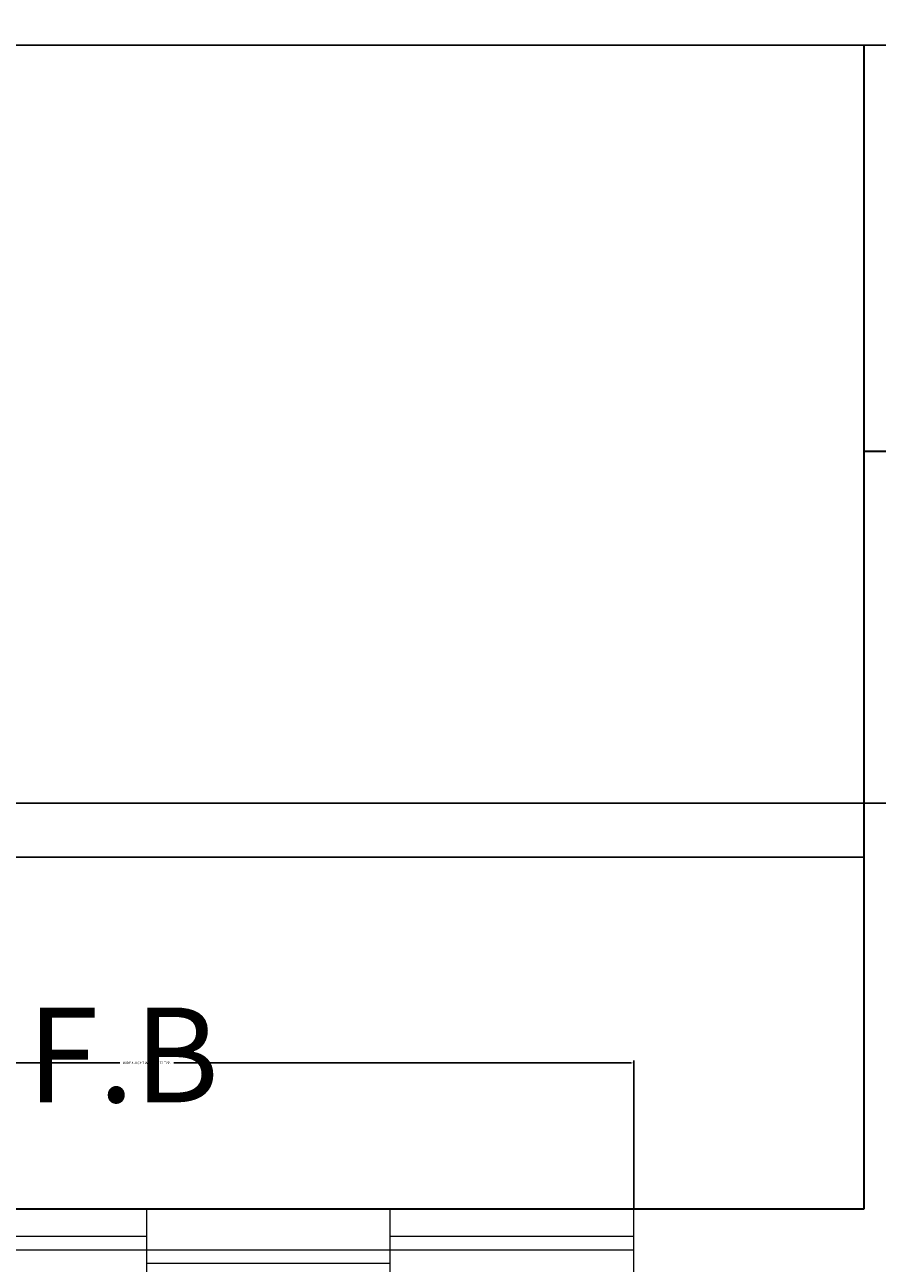
# Model space of a CAD drawing. Units: feet. Extents: x 105 to 1094, y -88 to 588.
# Tile 57 of 59: x 699 to 762, y 437 to 529. Entities that reach past the tile are written whole.
import ezdxf

# ---------------------------------------------------------------- set-up
doc = ezdxf.new("R2010")
doc.units = ezdxf.units.FT
doc.header["$MEASUREMENT"] = 0
for name, color, linetype, lineweight in [('A-ANNO-DIMS', 2, 'Continuous', 18), ('A-ANNO-TEXT', 7, 'Continuous', 18), ('A-FLOR-PROJ', 8, 'Continuous', 25), ('A-GLAZ', 4, 'Continuous', 18), ('A-WALL', 7, 'Continuous', 35)]:
    doc.layers.add(name, color=color, linetype=linetype, lineweight=lineweight)
doc.styles.get("Standard").update_dxf_attribs({"font": 'arial.ttf'})
doc.dimstyles.get("Standard").update_dxf_attribs({"dimtxt": 0.18, "dimasz": 0.18, "dimexe": 0.18, "dimexo": 0.0625, "dimgap": 0.09, "dimtad": 0, "dimtih": 1, "dimtoh": 1, "dimdec": 4, "dimzin": 0, "dimdsep": 46, "dimtxsty": 'Standard', "dimcen": 0.09, "dimadec": 0, "dimazin": 0, "dimtfac": 1, "dimtdec": 4, "dimtofl": 0, "dimtmove": 0, "dimatfit": 3, "dimfxl": 1, "dimtolj": 1, "dimtzin": 0, "dimarcsym": 0})

# ---------------------------------------------------------------- blocks, each defined once
blk = doc.blocks.new('WIN-FOUR-LIGHT-WIDE')
for p, q in [((0, 0), (0, 6)), ((18, 0), (18, 6)), ((36, 0), (36, 6)), ((54, 0), (54, 6)), ((72, 0), (72, 6)), ((18, 4), (36, 4)), ((54, 4), (72, 4)), ((0, 3), (72, 3)), ((0, 2), (18, 2)), ((36, 2), (54, 2))]:
    blk.add_line(p, q)
blk = doc.blocks.new('*D12')
at = {"layer": 'A-ANNO-DIMS', "color": 0, "lineweight": -2, "transparency": 16777216}
for p, q in [((671.688, 441.144), (671.688, 452.061)), ((671.868, 451.881), (705.69, 451.881)), ((743.508, 451.881), (709.687, 451.881)), ((743.688, 441.144), (743.688, 452.061))]:
    blk.add_line(p, q, dxfattribs=at)
at = {"layer": 'A-ANNO-DIMS', "color": 0, "transparency": 16777216}
for points in [[(671.868, 451.911), (671.868, 451.851), (671.688, 451.881)], [(743.508, 451.911), (743.508, 451.851), (743.688, 451.881)]]:
    blk.add_solid(points, dxfattribs=at)
at = {"layer": 'Defpoints', "color": 0, "transparency": 16777216}
for p in [(743.688, 451.881), (671.688, 441.081), (743.688, 441.081)]:
    blk.add_point(p, dxfattribs=at)
at = {"layer": 'A-ANNO-DIMS', "color": 0, "transparency": 16777216, "insert": (707.688, 451.881), "char_height": 0.18, "attachment_point": 5}
blk.add_mtext('\\A1;WIDE 4-LIGHT WINDOW 72 TYP.', dxfattribs=at)
blk = doc.blocks.new('*D21')
at = {"layer": 'A-ANNO-DIMS', "color": 0, "lineweight": -2, "transparency": 16777216}
for p, q in [((849.626, 543.081), (105.458, 543.081)), ((105.638, 542.901), (105.638, 250.263)), ((105.638, -42.739), (105.638, 249.899)), ((849.626, -42.919), (105.458, -42.919))]:
    blk.add_line(p, q, dxfattribs=at)
at = {"layer": 'A-ANNO-DIMS', "color": 0, "transparency": 16777216}
for points in [[(105.608, 542.901), (105.668, 542.901), (105.638, 543.081)], [(105.608, -42.739), (105.668, -42.739), (105.638, -42.919)]]:
    blk.add_solid(points, dxfattribs=at)
at = {"layer": 'Defpoints', "color": 0, "transparency": 16777216}
for p in [(105.638, 543.081), (849.688, 543.081), (849.688, -42.919)]:
    blk.add_point(p, dxfattribs=at)
at = {"layer": 'A-ANNO-DIMS', "color": 0, "transparency": 16777216, "insert": (105.638, 250.081), "char_height": 0.18, "attachment_point": 5}
blk.add_mtext('\\A1;586', dxfattribs=at)
blk = doc.blocks.new('*D30')
at = {"layer": 'A-ANNO-DIMS', "color": 0, "lineweight": -2, "transparency": 16777216}
for p, q in [((349.751, 543.081), (1093.918, 543.081)), ((1093.738, 542.901), (1093.738, 535.263)), ((1093.738, 527.261), (1093.738, 534.899)), ((349.751, 527.081), (1093.918, 527.081))]:
    blk.add_line(p, q, dxfattribs=at)
at = {"layer": 'A-ANNO-DIMS', "color": 0, "transparency": 16777216}
for points in [[(1093.708, 542.901), (1093.768, 542.901), (1093.738, 543.081)], [(1093.708, 527.261), (1093.768, 527.261), (1093.738, 527.081)]]:
    blk.add_solid(points, dxfattribs=at)
at = {"layer": 'Defpoints', "color": 0, "transparency": 16777216}
for p in [(349.688, 543.081), (349.688, 527.081), (1093.738, 527.081)]:
    blk.add_point(p, dxfattribs=at)
at = {"layer": 'A-ANNO-DIMS', "color": 0, "transparency": 16777216, "insert": (1093.738, 535.081), "char_height": 0.18, "attachment_point": 5}
blk.add_mtext('\\A1;16', dxfattribs=at)
blk = doc.blocks.new('*D31')
at = {"layer": 'A-ANNO-DIMS', "color": 0, "lineweight": -2, "transparency": 16777216}
for p, q in [((438.751, 527.081), (1093.918, 527.081)), ((1093.738, 526.901), (1093.738, 499.263)), ((1093.738, 471.261), (1093.738, 498.899)), ((438.751, 471.081), (1093.918, 471.081))]:
    blk.add_line(p, q, dxfattribs=at)
at = {"layer": 'A-ANNO-DIMS', "color": 0, "transparency": 16777216}
for points in [[(1093.708, 526.901), (1093.768, 526.901), (1093.738, 527.081)], [(1093.708, 471.261), (1093.768, 471.261), (1093.738, 471.081)]]:
    blk.add_solid(points, dxfattribs=at)
at = {"layer": 'Defpoints', "color": 0, "transparency": 16777216}
for p in [(438.688, 527.081), (1093.738, 527.081), (438.688, 471.081)]:
    blk.add_point(p, dxfattribs=at)
at = {"layer": 'A-ANNO-DIMS', "color": 0, "transparency": 16777216, "insert": (1093.738, 499.081), "char_height": 0.18, "attachment_point": 5}
blk.add_mtext('\\A1;56', dxfattribs=at)

msp = doc.modelspace()

# ---------------------------------------------------------------- linework, layer by layer
at = {"layer": 'A-FLOR-PROJ'}
for p, q in [((760.6883, 527.0812), (849.6883, 527.0812)), ((760.6883, 471.0812), (646.6883, 471.0812)), ((760.6883, 467.0812), (650.6883, 467.0812))]:
    msp.add_line(p, q, dxfattribs=at)
at = {"layer": 'A-WALL'}
for p, q in [((760.6883, 527.0812), (760.6883, 441.0812)), ((760.6883, 497.0812), (849.6883, 497.0812)), ((760.6883, 441.0812), (646.6883, 441.0812))]:
    msp.add_line(p, q, dxfattribs=at)

# ---------------------------------------------------------------- block references
at = {"layer": 'A-GLAZ'}
msp.add_blockref('WIN-FOUR-LIGHT-WIDE', (671.688, 435.081), dxfattribs=at)

# ---------------------------------------------------------------- texts
at = {"layer": 'A-ANNO-TEXT', "insert": (656.7611, 455.9748), "char_height": 7, "attachment_point": 1}
msp.add_mtext_dynamic_manual_height_columns('\\pxqc;F.B ', width=98.34246, gutter_width=1, heights=[0], dxfattribs=at)

# ---------------------------------------------------------------- dimensions: what is measured, and where the dimension line sits
at = {"layer": 'A-ANNO-DIMS'}
for base, p1, p2, picture, middle in [((105.6383, 543.0812), (849.6883, -42.9188), (849.6883, 543.0812), '*D21', (105.6383, 250.0812)), ((1093.7383, 527.0812), (349.6883, 543.0812), (349.6883, 527.0812), '*D30', (1093.7383, 535.0812)), ((1093.7383, 527.0812), (438.6883, 471.0812), (438.6883, 527.0812), '*D31', (1093.7383, 499.0812))]:
    dim = msp.add_linear_dim(base=base, p1=p1, p2=p2, angle=90, dimstyle='Standard', override={"dimdec": 0, "dimlfac": 1, "dimrnd": 0, "dimzin": 0, "dimdsep": 46, "dimlunit": 2}, dxfattribs=at)
    dim.commit()
    dim.dimension.update_dxf_attribs({"geometry": picture, "text_midpoint": middle})
dim = msp.add_linear_dim(base=(743.6883, 451.8812), p1=(671.6883, 441.0812), p2=(743.6883, 441.0812), text='WIDE 4-LIGHT WINDOW <> TYP.', dimstyle='Standard', override={"dimdec": 0, "dimlfac": 1, "dimrnd": 0, "dimzin": 0, "dimdsep": 46, "dimlunit": 2}, dxfattribs=at)
dim.commit()
dim.dimension.update_dxf_attribs({"geometry": '*D12', "text_midpoint": (707.6883, 451.8812)})

doc.saveas('drawing.dxf')
